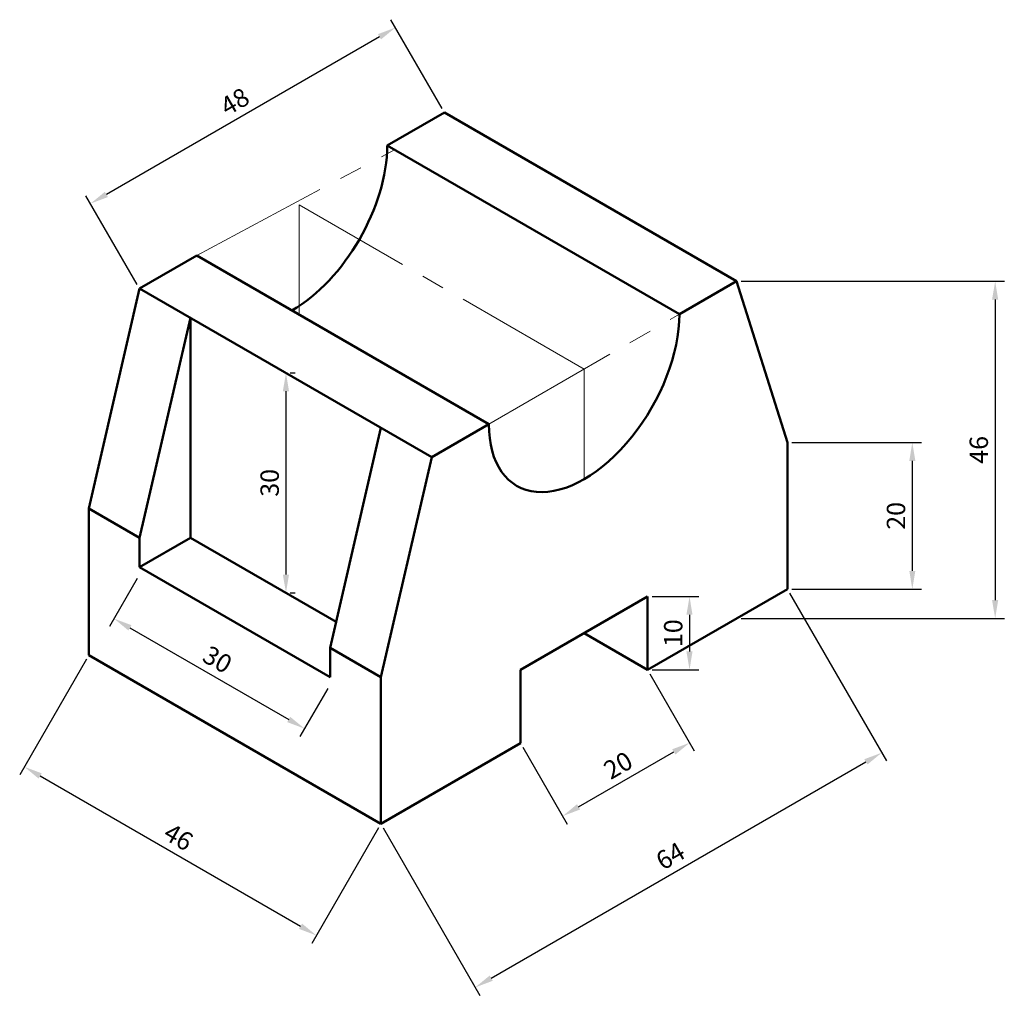
# Model space of a CAD drawing. Units: millimetres. Extents: x 985 to 1119, y 630 to 763.
import ezdxf

# ---------------------------------------------------------------- set-up
doc = ezdxf.new("R2010")
doc.units = ezdxf.units.MM
doc.linetypes.add('CENTER2', pattern=[28.575, 19.05, -3.175, 3.175, -3.175])
for name, color, linetype, lineweight in [('M-CNTR', 1, 'CENTER2', 18), ('M-DIMS', 2, 'Continuous', 25), ('M-OUTL', 7, 'Continuous', 50)]:
    doc.layers.add(name, color=color, linetype=linetype, lineweight=lineweight)
doc.styles.get("Standard").update_dxf_attribs({"font": 'arial.ttf'})
doc.dimstyles.new('ISO-25', dxfattribs={"dimtxt": 2.5, "dimasz": 2.5, "dimexe": 1.25, "dimexo": 0.625, "dimtad": 1, "dimtxsty": 'Standard', "dimcen": 2.5, "dimadec": 0, "dimazin": 0, "dimtfac": 1, "dimtmove": 0, "dimatfit": 3, "dimfxl": 1, "dimarcsym": 0})

# ---------------------------------------------------------------- blocks, each defined once
blk = doc.blocks.new('*D1')
at = {"layer": 'Defpoints', "color": 0, "transparency": 16777216}
for p in [(994.29, 676.17), (1034.12, 653.17), (1025.33, 637.95)]:
    blk.add_point(p, dxfattribs=at)
at = {"layer": 'M-DIMS', "color": 0, "lineweight": -2, "transparency": 16777216}
for p, q in [((993.97, 675.63), (984.87, 659.86)), ((987.66, 659.7), (1023.17, 639.2)), ((1033.81, 652.63), (1024.71, 636.86))]:
    blk.add_line(p, q, dxfattribs=at)
at = {"layer": 'M-DIMS', "color": 0, "transparency": 16777216}
for points in [[(987.87, 660.06), (987.45, 659.34), (985.5, 660.95)], [(1023.38, 639.56), (1022.96, 638.84), (1025.33, 637.95)]]:
    blk.add_solid(points, dxfattribs=at)
at = {"layer": 'M-DIMS', "color": 0, "transparency": 16777216, "insert": (1006.37, 651.09), "char_height": 2.5, "attachment_point": 5, "rotation": 330}
blk.add_mtext('46', dxfattribs=at)
blk = doc.blocks.new('*D2')
at = {"layer": 'Defpoints', "color": 0, "transparency": 16777216}
for p in [(1082.62, 727.17), (1082.62, 681.17), (1117.89, 681.17)]:
    blk.add_point(p, dxfattribs=at)
at = {"layer": 'M-DIMS', "color": 0, "lineweight": -2, "transparency": 16777216}
for p, q in [((1083.25, 727.17), (1119.14, 727.17)), ((1117.89, 724.67), (1117.89, 683.67)), ((1083.25, 681.17), (1119.14, 681.17))]:
    blk.add_line(p, q, dxfattribs=at)
at = {"layer": 'M-DIMS', "color": 0, "transparency": 16777216}
for points in [[(1117.47, 724.67), (1118.3, 724.67), (1117.89, 727.17)], [(1117.47, 683.67), (1118.3, 683.67), (1117.89, 681.17)]]:
    blk.add_solid(points, dxfattribs=at)
at = {"layer": 'M-DIMS', "color": 0, "transparency": 16777216, "insert": (1115.98, 704.17), "char_height": 2.5, "attachment_point": 5, "rotation": 90}
blk.add_mtext('46', dxfattribs=at)
blk = doc.blocks.new('*D3')
at = {"layer": 'Defpoints', "color": 0, "transparency": 16777216}
for p in [(1089.55, 705.17), (1089.55, 685.17), (1106.59, 685.17)]:
    blk.add_point(p, dxfattribs=at)
at = {"layer": 'M-DIMS', "color": 0, "lineweight": -2, "transparency": 16777216}
for p, q in [((1090.17, 705.17), (1107.84, 705.17)), ((1106.59, 702.67), (1106.59, 687.67)), ((1090.17, 685.17), (1107.84, 685.17))]:
    blk.add_line(p, q, dxfattribs=at)
at = {"layer": 'M-DIMS', "color": 0, "transparency": 16777216}
for points in [[(1106.18, 702.67), (1107.01, 702.67), (1106.59, 705.17)], [(1106.18, 687.67), (1107.01, 687.67), (1106.59, 685.17)]]:
    blk.add_solid(points, dxfattribs=at)
at = {"layer": 'M-DIMS', "color": 0, "transparency": 16777216, "insert": (1104.69, 695.17), "char_height": 2.5, "attachment_point": 5, "rotation": 90}
blk.add_mtext('20', dxfattribs=at)
blk = doc.blocks.new('*D4')
at = {"layer": 'Defpoints', "color": 0, "transparency": 16777216}
for p in [(1001.21, 687.17), (1027.2, 672.17), (1023.72, 666.15)]:
    blk.add_point(p, dxfattribs=at)
at = {"layer": 'M-DIMS', "color": 0, "lineweight": -2, "transparency": 16777216}
for p, q in [((1000.9, 686.63), (997.11, 680.07)), ((999.9, 679.9), (1021.55, 667.4)), ((1026.88, 671.63), (1023.09, 665.07))]:
    blk.add_line(p, q, dxfattribs=at)
at = {"layer": 'M-DIMS', "color": 0, "transparency": 16777216}
for points in [[(1000.11, 680.26), (999.69, 679.54), (997.74, 681.15)], [(1021.76, 667.76), (1021.35, 667.04), (1023.72, 666.15)]]:
    blk.add_solid(points, dxfattribs=at)
at = {"layer": 'M-DIMS', "color": 0, "transparency": 16777216, "insert": (1011.68, 675.3), "char_height": 2.5, "attachment_point": 5, "rotation": 330}
blk.add_mtext('30', dxfattribs=at)
blk = doc.blocks.new('*D5')
at = {"layer": 'Defpoints', "color": 0, "transparency": 16777216}
for p in [(1021.13, 714.67), (1021.13, 684.67), (1021.18, 684.67)]:
    blk.add_point(p, dxfattribs=at)
at = {"layer": 'M-DIMS', "color": 0, "lineweight": -2, "transparency": 16777216}
for p, q in [((1021.76, 714.67), (1022.43, 714.67)), ((1021.18, 712.17), (1021.18, 687.17)), ((1021.76, 684.67), (1022.43, 684.67))]:
    blk.add_line(p, q, dxfattribs=at)
at = {"layer": 'M-DIMS', "color": 0, "transparency": 16777216}
for points in [[(1020.76, 712.17), (1021.6, 712.17), (1021.18, 714.67)], [(1020.76, 687.17), (1021.6, 687.17), (1021.18, 684.67)]]:
    blk.add_solid(points, dxfattribs=at)
at = {"layer": 'M-DIMS', "color": 0, "transparency": 16777216, "insert": (1019.28, 699.67), "char_height": 2.5, "attachment_point": 5, "rotation": 90}
blk.add_mtext('30', dxfattribs=at)
blk = doc.blocks.new('*D6')
at = {"layer": 'Defpoints', "color": 0, "transparency": 16777216}
for p in [(1042.78, 750.17), (994.53, 737.75), (1001.21, 726.17)]:
    blk.add_point(p, dxfattribs=at)
at = {"layer": 'M-DIMS', "color": 0, "lineweight": -2, "transparency": 16777216}
for p, q in [((1042.47, 750.71), (1035.48, 762.83)), ((1033.94, 760.5), (996.7, 739)), ((1000.9, 726.71), (993.91, 738.83))]:
    blk.add_line(p, q, dxfattribs=at)
at = {"layer": 'M-DIMS', "color": 0, "transparency": 16777216}
for points in [[(1033.73, 760.86), (1034.14, 760.14), (1036.1, 761.75)], [(996.49, 739.36), (996.9, 738.64), (994.53, 737.75)]]:
    blk.add_solid(points, dxfattribs=at)
at = {"layer": 'M-DIMS', "color": 0, "transparency": 16777216, "insert": (1014.36, 751.39), "char_height": 2.5, "attachment_point": 5, "rotation": 30}
blk.add_mtext('48', dxfattribs=at)
blk = doc.blocks.new('*D7')
at = {"layer": 'Defpoints', "color": 0, "transparency": 16777216}
for p in [(1070.5, 684.17), (1070.5, 674.17), (1076.21, 674.17)]:
    blk.add_point(p, dxfattribs=at)
at = {"layer": 'M-DIMS', "color": 0, "lineweight": -2, "transparency": 16777216}
for p, q in [((1071.12, 684.17), (1077.46, 684.17)), ((1076.21, 681.67), (1076.21, 676.67)), ((1071.12, 674.17), (1077.46, 674.17))]:
    blk.add_line(p, q, dxfattribs=at)
at = {"layer": 'M-DIMS', "color": 0, "transparency": 16777216}
for points in [[(1075.79, 681.67), (1076.62, 681.67), (1076.21, 684.17)], [(1075.79, 676.67), (1076.62, 676.67), (1076.21, 674.17)]]:
    blk.add_solid(points, dxfattribs=at)
at = {"layer": 'M-DIMS', "color": 0, "transparency": 16777216, "insert": (1074.31, 679.17), "char_height": 2.5, "attachment_point": 5, "rotation": 90}
blk.add_mtext('10', dxfattribs=at)
blk = doc.blocks.new('*D8')
at = {"layer": 'Defpoints', "color": 0, "transparency": 16777216}
for p in [(1089.55, 685.17), (1102.43, 662.87), (1034.12, 653.17)]:
    blk.add_point(p, dxfattribs=at)
at = {"layer": 'M-DIMS', "color": 0, "lineweight": -2, "transparency": 16777216}
for p, q in [((1089.86, 684.63), (1103.05, 661.78)), ((1049.17, 632.12), (1100.26, 661.62)), ((1034.44, 652.63), (1047.63, 629.78))]:
    blk.add_line(p, q, dxfattribs=at)
at = {"layer": 'M-DIMS', "color": 0, "transparency": 16777216}
for points in [[(1100.05, 661.98), (1100.47, 661.26), (1102.43, 662.87)], [(1048.96, 632.48), (1049.37, 631.76), (1047, 630.87)]]:
    blk.add_solid(points, dxfattribs=at)
at = {"layer": 'M-DIMS', "color": 0, "transparency": 16777216, "insert": (1073.76, 648.51), "char_height": 2.5, "attachment_point": 5, "rotation": 30}
blk.add_mtext('64', dxfattribs=at)
blk = doc.blocks.new('*D9')
at = {"layer": 'Defpoints', "color": 0, "transparency": 16777216}
for p in [(1070.5, 674.17), (1053.18, 664.17), (1076.24, 664.23)]:
    blk.add_point(p, dxfattribs=at)
at = {"layer": 'M-DIMS', "color": 0, "lineweight": -2, "transparency": 16777216}
for p, q in [((1070.81, 673.63), (1076.86, 663.14)), ((1053.49, 663.63), (1059.54, 653.14)), ((1061.08, 655.48), (1074.07, 662.98))]:
    blk.add_line(p, q, dxfattribs=at)
at = {"layer": 'M-DIMS', "color": 0, "transparency": 16777216}
for points in [[(1073.86, 663.34), (1074.28, 662.62), (1076.24, 664.23)], [(1060.87, 655.84), (1061.29, 655.12), (1058.92, 654.23)]]:
    blk.add_solid(points, dxfattribs=at)
at = {"layer": 'M-DIMS', "color": 0, "transparency": 16777216, "insert": (1066.63, 660.87), "char_height": 2.5, "attachment_point": 5, "rotation": 30}
blk.add_mtext('20', dxfattribs=at)

msp = doc.modelspace()

# ---------------------------------------------------------------- linework, layer by layer
at = {"layer": 'M-CNTR'}
for p, q in [((1009.009, 730.671), (1035.984, 745.097)), ((1061.836, 715.171), (1022.994, 737.597)), ((1022.994, 737.597), (1022.994, 722.597)), ((1048.846, 707.671), (1074.827, 722.671)), ((1061.836, 715.171), (1061.836, 700.171))]:
    msp.add_line(p, q, dxfattribs=at)
at = {"layer": 'M-OUTL'}
for p, q in [((1042.784, 750.171), (1034.99, 745.671)), ((1082.621, 727.171), (1042.784, 750.171)), ((1034.99, 745.671), (1074.827, 722.671)), ((1009.009, 730.671), (1001.215, 726.171)), ((1048.846, 707.671), (1009.009, 730.671)), ((1074.827, 722.671), (1082.621, 727.171)), ((1082.621, 727.171), (1089.549, 705.171)), ((994.286, 696.171), (1001.215, 726.171)), ((1041.052, 703.171), (1001.215, 726.171)), ((1008.143, 722.171), (1001.215, 692.171)), ((1008.143, 722.171), (1008.143, 692.171)), ((1048.846, 707.671), (1041.052, 703.171)), ((1034.124, 707.171), (1027.195, 677.171)), ((1089.549, 685.171), (1089.549, 705.171)), ((1034.124, 673.171), (1041.052, 703.171)), ((994.286, 676.171), (994.286, 696.171)), ((994.286, 696.171), (1001.215, 692.171)), ((1001.215, 688.171), (1001.215, 692.171)), ((1001.215, 688.171), (1008.143, 692.171)), ((1008.143, 692.171), (1028.01, 680.701)), ((1027.196, 673.171), (1001.215, 688.171)), ((1070.497, 674.171), (1089.549, 685.171)), ((1053.176, 674.171), (1070.497, 684.171)), ((1070.497, 684.171), (1070.497, 674.171)), ((1070.497, 674.171), (1061.837, 679.171)), ((1034.124, 673.171), (1027.195, 677.171)), ((1027.196, 673.171), (1027.196, 677.171)), ((994.286, 676.171), (1034.124, 653.171)), ((1053.176, 664.171), (1053.176, 674.171)), ((1034.124, 653.171), (1034.124, 673.171)), ((1034.124, 653.171), (1053.176, 664.171))]:
    msp.add_line(p, q, dxfattribs=at)
for centre, major_axis, start_param, end_param in [((1022, 738.171), (9.186, 15.91), 3.9269908, 5.4977871), ((1061.836, 715.171), (-9.186, -15.91), 5.4977871, 8.6393798)]:
    msp.add_ellipse(centre, major_axis=major_axis, ratio=0.5773503, start_param=start_param, end_param=end_param, dxfattribs=at)

# ---------------------------------------------------------------- dimensions: what is measured, and where the dimension line sits
at = {"layer": 'M-DIMS'}
for p1, p2, distance, picture, middle in [((1042.784, 750.171), (1001.215, 726.171), -13.367, '*D6', (1014.365, 751.394)), ((1082.621, 727.171), (1082.621, 681.171), 35.264, '*D2', (1115.984, 704.171)), ((1021.133, 714.671), (1021.133, 684.671), 0.045, '*D5', (1019.276, 699.671)), ((1001.215, 687.171), (1027.195, 672.171), -6.953, '*D4', (1011.68, 675.298)), ((1034.124, 653.171), (1089.549, 685.171), -25.756, '*D8', (1073.764, 648.513)), ((1070.497, 684.171), (1070.497, 674.171), 5.71, '*D7', (1074.305, 679.171)), ((994.286, 676.171), (1034.124, 653.171), -17.58, '*D1', (1006.366, 651.094)), ((1053.176, 664.171), (1070.497, 674.171), -11.483, '*D9', (1066.627, 660.874))]:
    dim = msp.add_aligned_dim(p1=p1, p2=p2, distance=distance, dimstyle='ISO-25', override={"dimclrd": 0, "dimclre": 0, "dimclrt": 0}, dxfattribs=at)
    dim.commit()
    dim.dimension.update_dxf_attribs({"geometry": picture, "text_midpoint": middle})
dim = msp.add_linear_dim(base=(1106.593, 685.171), p1=(1089.549, 705.171), p2=(1089.549, 685.171), angle=90, dimstyle='ISO-25', override={"dimclrd": 0, "dimclre": 0, "dimclrt": 0}, dxfattribs=at)
dim.commit()
dim.dimension.update_dxf_attribs({"geometry": '*D3', "text_midpoint": (1104.692, 695.171)})

doc.saveas('drawing.dxf')
